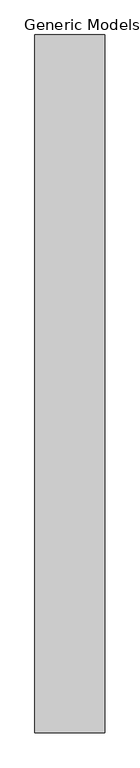
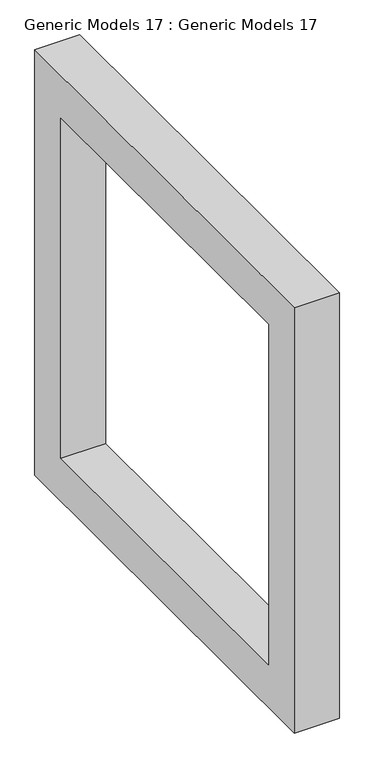
"""IFC4 building model written with IfcOpenShell, lengths in millimetres: proxy geometry, Generic Models 17 : Generic Models 17."""

from ifc_helpers import new_model, si_unit, frame, origin, place, context, project, spatial, polyline, outline, extrude, source, transform, mapped, element, save


def generic_models_17_generic_models_17_4194431e(model_context):
    return source(origin(), model_context, "Body", "SweptSolid", [
        extrude(outline(polyline([(-3005.5794704, 11734.8), (-1481.5794704, 11734.8), (-1481.5794704, 10210.8), (-3005.5794704, 10210.8), (-3005.5794704, 11734.8)]), holes=[polyline([(-2853.1794704, 11582.4), (-2853.1794704, 10363.2), (-1633.9794704, 10363.2), (-1633.9794704, 11582.4), (-2853.1794704, 11582.4)])]), frame((-15526.3456086, 0.0, 0.0), z_axis=(1.0, 0.0, 0.0), x_axis=(0.0, 1.0, 0.0)), (0.0, 0.0, 1.0), 152.4),
    ])


if __name__ == "__main__":
    model = new_model("IFC4")
    model_context = context("Model", 3, world=origin())
    ifc_project = project(units=[si_unit("LENGTHUNIT", "METRE", prefix="MILLI")], contexts=[model_context])
    site = spatial("IfcSite", under=ifc_project)
    building = spatial("IfcBuilding", under=site)
    placement = place(None, origin())
    generic_models_17_generic_models_17_shape = generic_models_17_generic_models_17_4194431e(model_context)
    element("IfcBuildingElementProxy", 1, Name="Generic Models 17 : Generic Models 17", ObjectType="Generic Models 17 : Generic Models 17", at=placement, inside=building, context=model_context, shape_type="MappedRepresentation", body=[
        mapped(generic_models_17_generic_models_17_shape, transform((0.0, 0.0, 0.0), x_axis=(1.0, 0.0, 0.0), y_axis=(0.0, 1.0, 0.0), z_axis=(0.0, 0.0, 1.0))),
    ])
    save(model, "model.ifc")

# Revit data of these elements
# Element 1 (IfcBuildingElementProxy, "Generic Models 17 : Generic Models 17")
#   Materials on its faces: "TEAK BROWN COLOUR"
# Materials
#   "TEAK BROWN COLOUR": class "Generic", colour RGB 120 120 120, transparency 0, Cost = 0
